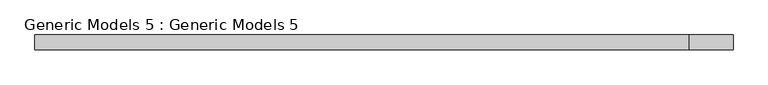
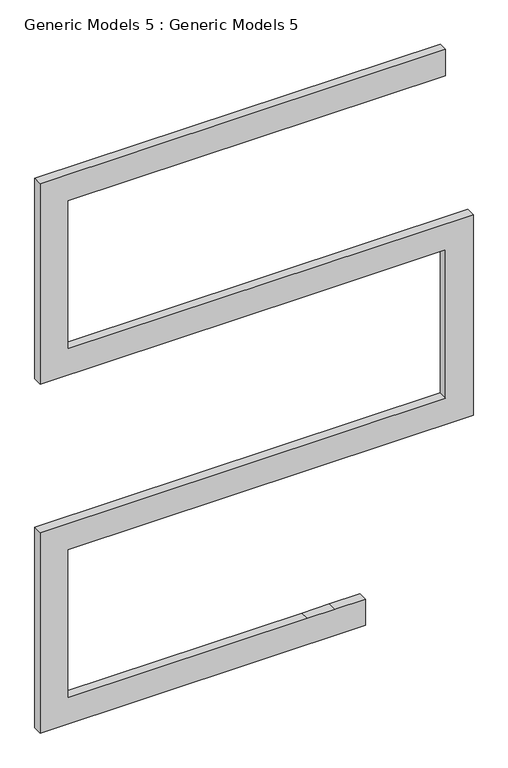
"""IFC4 building model written with IfcOpenShell, lengths in millimetres: proxy geometry, Generic Models 5 : Generic Models 5."""

from ifc_helpers import new_model, si_unit, frame, origin, place, context, project, spatial, polyline, outline, extrude, source, transform, mapped, element, save


def generic_models_5_generic_models_5_4128d2ba(model_context):
    return source(origin(), model_context, "Body", "SweptSolid", [
        extrude(outline(polyline([(9448.8, -10192.3456086), (5943.6, -10192.3456086), (5943.6, -5772.7456086), (5943.6, -3486.7456086), (3352.8, -3486.7456086), (3352.8, -10192.3456086), (-152.4, -10192.3456086), (-152.4, -4813.6091294), (304.8, -4813.6091294), (304.8, -5315.5456086), (304.8, -5772.7456086), (304.8, -9735.1456086), (2895.6, -9735.1456086), (2895.6, -3029.5456086), (6400.8, -3029.5456086), (6400.8, -9735.1456086), (8991.6, -9735.1456086), (8991.6, -3486.7456086), (9448.8, -3486.7456086), (9448.8, -10192.3456086)])), frame((0.0, -11268.8679047, 0.0), z_axis=(0.0, 1.0, 0.0), x_axis=(0.0, 0.0, 1.0)), (0.0, 0.0, 1.0), 152.4),
    ])


if __name__ == "__main__":
    model = new_model("IFC4")
    model_context = context("Model", 3, world=origin())
    ifc_project = project(units=[si_unit("LENGTHUNIT", "METRE", prefix="MILLI")], contexts=[model_context])
    site = spatial("IfcSite", under=ifc_project)
    building = spatial("IfcBuilding", under=site)
    placement = place(None, origin())
    generic_models_5_generic_models_5_shape = generic_models_5_generic_models_5_4128d2ba(model_context)
    element("IfcBuildingElementProxy", 1, Name="Generic Models 5 : Generic Models 5", ObjectType="Generic Models 5 : Generic Models 5", at=placement, inside=building, context=model_context, shape_type="MappedRepresentation", body=[
        mapped(generic_models_5_generic_models_5_shape, transform((0.0, 0.0, 0.0), x_axis=(1.0, 0.0, 0.0), y_axis=(0.0, 1.0, 0.0), z_axis=(0.0, 0.0, 1.0))),
    ])
    save(model, "model.ifc")

# Revit data of these elements
# Element 1 (IfcBuildingElementProxy, "Generic Models 5 : Generic Models 5")
#   Materials on its faces: "WALL ACCENT 6\""
# Materials
#   "WALL ACCENT 6\"": class "Generic", colour RGB 120 120 120, transparency 0, Cost = 0
